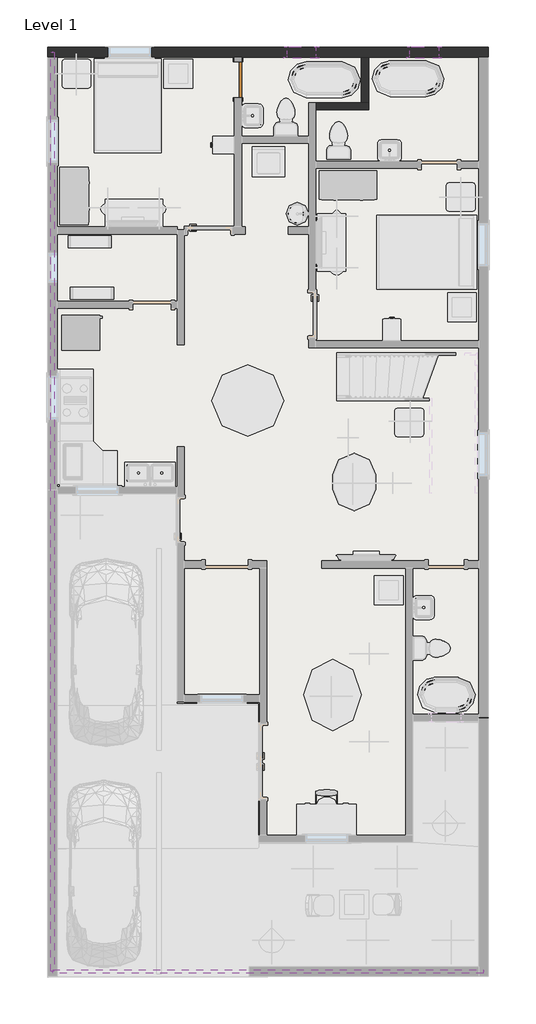
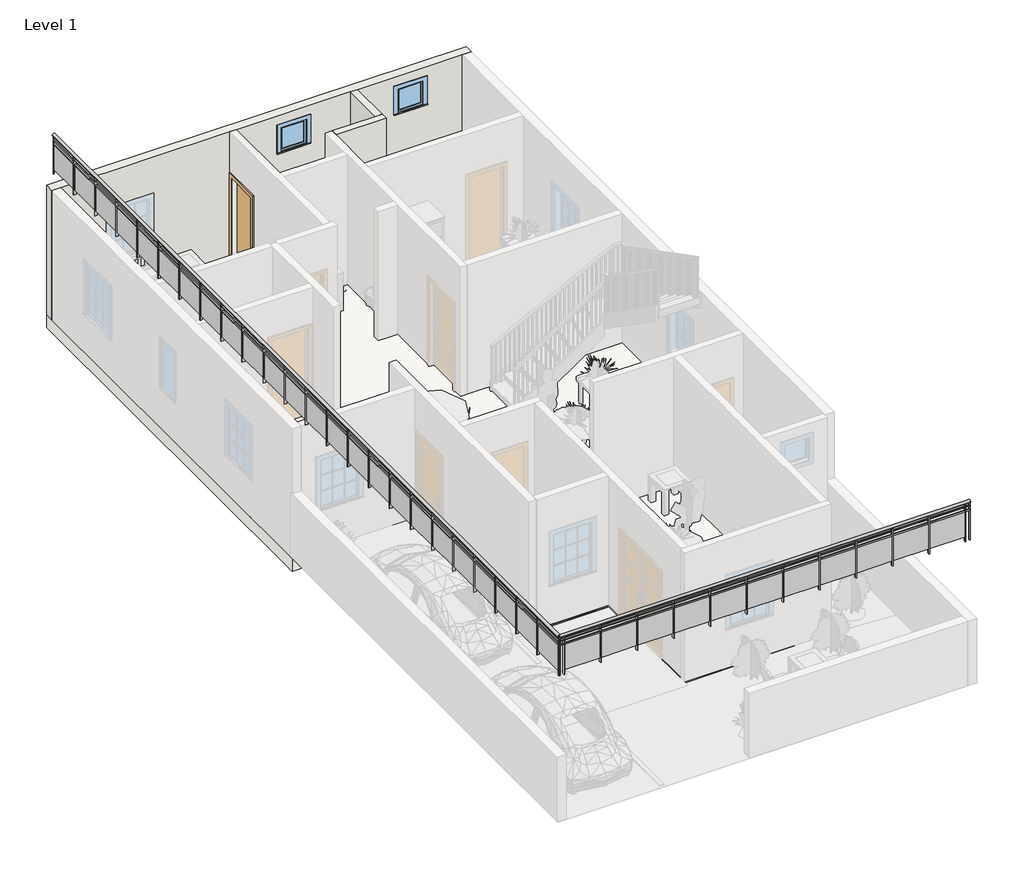
# One storey, part 2 of 4: 3 walls, 2 railings, 2 windows, 1 door, 1 slab.
"""IFC4 building model written with IfcOpenShell, lengths in millimetres."""

from ifc_helpers import new_model, si_unit, point, frame, origin, origin_with_axes, place, context, project, spatial, polyline, ellipse_curve, trimmed, outline, extrude, faceted_brep, transform, mapped, element, save
from ifc_brep_helpers import plane_surface, extruded_surface, advanced_brep
from components import door_255cab33, window_e41d21a6

model = new_model("IFC4")

# Units and contexts
model_context = context("Model", 3, world=origin())
ifc_project = project(units=[si_unit("LENGTHUNIT", "METRE", prefix="MILLI")], contexts=[model_context])

# Site, building, storey
site = spatial("IfcSite", under=ifc_project)
building = spatial("IfcBuilding", under=site)
storey = spatial("IfcBuildingStorey", under=building, Name="Level 1", Elevation=0.0)

# Door
placement = place(None, origin())
door_shape = door_255cab33(model_context)
element("IfcDoor", 1, ObjectType="Single-Flush : 30\" x 80\"", at=placement, inside=storey, context=model_context, shape_type="MappedRepresentation", body=[
    mapped(door_shape, transform((-7763.4976606, 13167.4271763, 0.0), x_axis=(0.0, 1.0, 0.0), y_axis=(-1.0, 0.0, 0.0), z_axis=(0.0, 0.0, 1.0))),
])

# Railings
element("IfcRailing", 2, ObjectType="Glass Panel - Bottom Fill", at=placement, inside=storey, context=model_context, shape_type="SolidModel", body=[
    advanced_brep(
    [(-2556.4976606, -5793.6728237, 4267.2), (-2556.4976606, -5717.4728237, 4267.2), (-11700.4976606, -5793.6728237, 4267.2), (-11700.4976606, -5717.4728237, 4267.2)],
    [
        (0, 1, ellipse_curve(frame((-2556.4976606, -5755.5728237, 4267.2), z_axis=(1.0, 0.0, 0.0), x_axis=(0.0, 1.0, 0.0)), 38.1, 28.575)),
        (1, 0, ellipse_curve(frame((-2556.4976606, -5755.5728237, 4267.2), z_axis=(1.0, 0.0, 0.0), x_axis=(0.0, 1.0, 0.0)), 38.1, 28.575)),
        (2, 3, ellipse_curve(frame((-11700.4976606, -5755.5728237, 4267.2), z_axis=(-1.0, 0.0, 0.0), x_axis=(0.0, 1.0, 0.0)), 38.1, 28.575)),
        (3, 2, ellipse_curve(frame((-11700.4976606, -5755.5728237, 4267.2), z_axis=(-1.0, 0.0, 0.0), x_axis=(0.0, 1.0, 0.0)), 38.1, 28.575)),
        (0, 2),
        (3, 1),
    ],
    [
        plane_surface(frame((-2556.4976606, -5755.5728237, 4267.2), z_axis=(1.0, 0.0, 0.0), x_axis=(0.0, -1.0, 0.0))),
        plane_surface(frame((-11700.4976606, -5755.5728237, 4267.2), z_axis=(-1.0, 0.0, 0.0), x_axis=(0.0, -1.0, 0.0))),
        extruded_surface(trimmed(ellipse_curve(frame((-11700.4976606, -5755.5728237, 4267.2), z_axis=(1.0, 0.0, 0.0), x_axis=(0.0, 1.0, 0.0)), 38.1, 28.575), [point((-11700.4976606, -5793.6728237, 4267.2))], [point((-11700.4976606, -5717.4728237, 4267.2))], True, "CARTESIAN"), (9144.0, 0.0, 0.0), 9144.0),
        extruded_surface(trimmed(ellipse_curve(frame((-11700.4976606, -5755.5728237, 4267.2), z_axis=(1.0, 0.0, 0.0), x_axis=(0.0, 1.0, 0.0)), 38.1, 28.575), [point((-11700.4976606, -5717.4728237, 4267.2))], [point((-11700.4976606, -5793.6728237, 4267.2))], True, "CARTESIAN"), (9144.0, 0.0, 0.0), 9144.0),
    ],
    [
        (0, [[1, 2]]),
        (1, [[3, 4]]),
        (2, [[-1, 5, -4, 6]]),
        (3, [[-2, -6, -3, -5]]),
    ],
),
    extrude(outline(polyline([(-2556.4976606, -5742.8728237), (-2556.4976606, -5768.2728237), (-11700.4976606, -5768.2728237), (-11700.4976606, -5742.8728237), (-2556.4976606, -5742.8728237)])), frame((0.0, 0.0, 4152.9), z_axis=(0.0, 0.0, 1.0), x_axis=(1.0, 0.0, 0.0)), (0.0, 0.0, 1.0), 25.4),
    extrude(outline(polyline([(-2556.4976606, -5742.8728237), (-2556.4976606, -5768.2728237), (-11700.4976606, -5768.2728237), (-11700.4976606, -5742.8728237), (-2556.4976606, -5742.8728237)])), frame((0.0, 0.0, 4051.3), z_axis=(0.0, 0.0, 1.0), x_axis=(1.0, 0.0, 0.0)), (0.0, 0.0, 1.0), 25.4),
    extrude(outline(polyline([(-11592.5476606, -5730.1728237), (-11592.5476606, -5780.9728237), (-11605.2476606, -5780.9728237), (-11605.2476606, -5730.1728237), (-11592.5476606, -5730.1728237)])), frame((0.0, 0.0, 3352.8), z_axis=(0.0, 0.0, 1.0), x_axis=(1.0, 0.0, 0.0)), (0.0, 0.0, 1.0), 885.6788223),
    extrude(outline(polyline([(-10786.0976606, -5762.1079807), (-11598.8976606, -5762.1079807), (-11598.8976606, -5755.7579807), (-10786.0976606, -5755.7579807), (-10786.0976606, -5762.1079807)])), frame((0.0, 0.0, 3454.4), z_axis=(0.0, 0.0, 1.0), x_axis=(1.0, 0.0, 0.0)), (0.0, 0.0, 1.0), 596.9),
    extrude(outline(polyline([(-10779.7476606, -5730.1728237), (-10779.7476606, -5780.9728237), (-10792.4476606, -5780.9728237), (-10792.4476606, -5730.1728237), (-10779.7476606, -5730.1728237)])), frame((0.0, 0.0, 3352.8), z_axis=(0.0, 0.0, 1.0), x_axis=(1.0, 0.0, 0.0)), (0.0, 0.0, 1.0), 885.6788223),
    extrude(outline(polyline([(-9973.2976606, -5762.1079807), (-10786.0976606, -5762.1079807), (-10786.0976606, -5755.7579807), (-9973.2976606, -5755.7579807), (-9973.2976606, -5762.1079807)])), frame((0.0, 0.0, 3454.4), z_axis=(0.0, 0.0, 1.0), x_axis=(1.0, 0.0, 0.0)), (0.0, 0.0, 1.0), 596.9),
    extrude(outline(polyline([(-9966.9476606, -5730.1728237), (-9966.9476606, -5780.9728237), (-9979.6476606, -5780.9728237), (-9979.6476606, -5730.1728237), (-9966.9476606, -5730.1728237)])), frame((0.0, 0.0, 3352.8), z_axis=(0.0, 0.0, 1.0), x_axis=(1.0, 0.0, 0.0)), (0.0, 0.0, 1.0), 885.6788223),
    extrude(outline(polyline([(-9160.4976606, -5762.1079807), (-9973.2976606, -5762.1079807), (-9973.2976606, -5755.7579807), (-9160.4976606, -5755.7579807), (-9160.4976606, -5762.1079807)])), frame((0.0, 0.0, 3454.4), z_axis=(0.0, 0.0, 1.0), x_axis=(1.0, 0.0, 0.0)), (0.0, 0.0, 1.0), 596.9),
    extrude(outline(polyline([(-9154.1476606, -5730.1728237), (-9154.1476606, -5780.9728237), (-9166.8476606, -5780.9728237), (-9166.8476606, -5730.1728237), (-9154.1476606, -5730.1728237)])), frame((0.0, 0.0, 3352.8), z_axis=(0.0, 0.0, 1.0), x_axis=(1.0, 0.0, 0.0)), (0.0, 0.0, 1.0), 885.6788223),
    extrude(outline(polyline([(-8347.6976606, -5762.1079807), (-9160.4976606, -5762.1079807), (-9160.4976606, -5755.7579807), (-8347.6976606, -5755.7579807), (-8347.6976606, -5762.1079807)])), frame((0.0, 0.0, 3454.4), z_axis=(0.0, 0.0, 1.0), x_axis=(1.0, 0.0, 0.0)), (0.0, 0.0, 1.0), 596.9),
    extrude(outline(polyline([(-8341.3476606, -5730.1728237), (-8341.3476606, -5780.9728237), (-8354.0476606, -5780.9728237), (-8354.0476606, -5730.1728237), (-8341.3476606, -5730.1728237)])), frame((0.0, 0.0, 3352.8), z_axis=(0.0, 0.0, 1.0), x_axis=(1.0, 0.0, 0.0)), (0.0, 0.0, 1.0), 885.6788223),
    extrude(outline(polyline([(-7534.8976606, -5762.1079807), (-8347.6976606, -5762.1079807), (-8347.6976606, -5755.7579807), (-7534.8976606, -5755.7579807), (-7534.8976606, -5762.1079807)])), frame((0.0, 0.0, 3454.4), z_axis=(0.0, 0.0, 1.0), x_axis=(1.0, 0.0, 0.0)), (0.0, 0.0, 1.0), 596.9),
    extrude(outline(polyline([(-7528.5476606, -5730.1728237), (-7528.5476606, -5780.9728237), (-7541.2476606, -5780.9728237), (-7541.2476606, -5730.1728237), (-7528.5476606, -5730.1728237)])), frame((0.0, 0.0, 3352.8), z_axis=(0.0, 0.0, 1.0), x_axis=(1.0, 0.0, 0.0)), (0.0, 0.0, 1.0), 885.6788223),
    extrude(outline(polyline([(-6722.0976606, -5762.1079807), (-7534.8976606, -5762.1079807), (-7534.8976606, -5755.7579807), (-6722.0976606, -5755.7579807), (-6722.0976606, -5762.1079807)])), frame((0.0, 0.0, 3454.4), z_axis=(0.0, 0.0, 1.0), x_axis=(1.0, 0.0, 0.0)), (0.0, 0.0, 1.0), 596.9),
    extrude(outline(polyline([(-6715.7476606, -5730.1728237), (-6715.7476606, -5780.9728237), (-6728.4476606, -5780.9728237), (-6728.4476606, -5730.1728237), (-6715.7476606, -5730.1728237)])), frame((0.0, 0.0, 3352.8), z_axis=(0.0, 0.0, 1.0), x_axis=(1.0, 0.0, 0.0)), (0.0, 0.0, 1.0), 885.6788223),
    extrude(outline(polyline([(-5909.2976606, -5762.1079807), (-6722.0976606, -5762.1079807), (-6722.0976606, -5755.7579807), (-5909.2976606, -5755.7579807), (-5909.2976606, -5762.1079807)])), frame((0.0, 0.0, 3454.4), z_axis=(0.0, 0.0, 1.0), x_axis=(1.0, 0.0, 0.0)), (0.0, 0.0, 1.0), 596.9),
    extrude(outline(polyline([(-5902.9476606, -5730.1728237), (-5902.9476606, -5780.9728237), (-5915.6476606, -5780.9728237), (-5915.6476606, -5730.1728237), (-5902.9476606, -5730.1728237)])), frame((0.0, 0.0, 3352.8), z_axis=(0.0, 0.0, 1.0), x_axis=(1.0, 0.0, 0.0)), (0.0, 0.0, 1.0), 885.6788223),
    extrude(outline(polyline([(-5096.4976606, -5762.1079807), (-5909.2976606, -5762.1079807), (-5909.2976606, -5755.7579807), (-5096.4976606, -5755.7579807), (-5096.4976606, -5762.1079807)])), frame((0.0, 0.0, 3454.4), z_axis=(0.0, 0.0, 1.0), x_axis=(1.0, 0.0, 0.0)), (0.0, 0.0, 1.0), 596.9),
    extrude(outline(polyline([(-5090.1476606, -5730.1728237), (-5090.1476606, -5780.9728237), (-5102.8476606, -5780.9728237), (-5102.8476606, -5730.1728237), (-5090.1476606, -5730.1728237)])), frame((0.0, 0.0, 3352.8), z_axis=(0.0, 0.0, 1.0), x_axis=(1.0, 0.0, 0.0)), (0.0, 0.0, 1.0), 885.6788223),
    extrude(outline(polyline([(-4283.6976606, -5762.1079807), (-5096.4976606, -5762.1079807), (-5096.4976606, -5755.7579807), (-4283.6976606, -5755.7579807), (-4283.6976606, -5762.1079807)])), frame((0.0, 0.0, 3454.4), z_axis=(0.0, 0.0, 1.0), x_axis=(1.0, 0.0, 0.0)), (0.0, 0.0, 1.0), 596.9),
    extrude(outline(polyline([(-4277.3476606, -5730.1728237), (-4277.3476606, -5780.9728237), (-4290.0476606, -5780.9728237), (-4290.0476606, -5730.1728237), (-4277.3476606, -5730.1728237)])), frame((0.0, 0.0, 3352.8), z_axis=(0.0, 0.0, 1.0), x_axis=(1.0, 0.0, 0.0)), (0.0, 0.0, 1.0), 885.6788223),
    extrude(outline(polyline([(-3470.8976606, -5762.1079807), (-4283.6976606, -5762.1079807), (-4283.6976606, -5755.7579807), (-3470.8976606, -5755.7579807), (-3470.8976606, -5762.1079807)])), frame((0.0, 0.0, 3454.4), z_axis=(0.0, 0.0, 1.0), x_axis=(1.0, 0.0, 0.0)), (0.0, 0.0, 1.0), 596.9),
    extrude(outline(polyline([(-3464.5476606, -5730.1728237), (-3464.5476606, -5780.9728237), (-3477.2476606, -5780.9728237), (-3477.2476606, -5730.1728237), (-3464.5476606, -5730.1728237)])), frame((0.0, 0.0, 3352.8), z_axis=(0.0, 0.0, 1.0), x_axis=(1.0, 0.0, 0.0)), (0.0, 0.0, 1.0), 885.6788223),
    extrude(outline(polyline([(-2658.0976606, -5762.1079807), (-3470.8976606, -5762.1079807), (-3470.8976606, -5755.7579807), (-2658.0976606, -5755.7579807), (-2658.0976606, -5762.1079807)])), frame((0.0, 0.0, 3454.4), z_axis=(0.0, 0.0, 1.0), x_axis=(1.0, 0.0, 0.0)), (0.0, 0.0, 1.0), 596.9),
    extrude(outline(polyline([(-2651.7476606, -5730.1728237), (-2651.7476606, -5780.9728237), (-2664.4476606, -5780.9728237), (-2664.4476606, -5730.1728237), (-2651.7476606, -5730.1728237)])), frame((0.0, 0.0, 3352.8), z_axis=(0.0, 0.0, 1.0), x_axis=(1.0, 0.0, 0.0)), (0.0, 0.0, 1.0), 885.6788223),
    extrude(outline(polyline([(-11687.7976606, -5746.0478237), (-11687.7976606, -5765.0978237), (-11706.8476606, -5765.0978237), (-11706.8476606, -5746.0478237), (-11687.7976606, -5746.0478237)])), frame((0.0, 0.0, 3352.8), z_axis=(0.0, 0.0, 1.0), x_axis=(1.0, 0.0, 0.0)), (0.0, 0.0, 1.0), 885.6788223),
    extrude(outline(polyline([(-2550.1476606, -5746.0478237), (-2550.1476606, -5765.0978237), (-2569.1976606, -5765.0978237), (-2569.1976606, -5746.0478237), (-2550.1476606, -5746.0478237)])), frame((0.0, 0.0, 3352.8), z_axis=(0.0, 0.0, 1.0), x_axis=(1.0, 0.0, 0.0)), (0.0, 0.0, 1.0), 885.6788223),
])
element("IfcRailing", 3, ObjectType="Glass Panel - Bottom Fill", at=placement, inside=storey, context=model_context, shape_type="SolidModel", body=[
    advanced_brep(
    [(-11738.5976606, -5755.5728237, 4267.2), (-11662.3976606, -5755.5728237, 4267.2), (-11738.5976606, 13751.6271763, 4267.2), (-11662.3976606, 13751.6271763, 4267.2)],
    [
        (0, 1, ellipse_curve(frame((-11700.4976606, -5755.5728237, 4267.2), z_axis=(0.0, -1.0, 0.0), x_axis=(1.0, 0.0, 0.0)), 38.1, 28.575)),
        (1, 0, ellipse_curve(frame((-11700.4976606, -5755.5728237, 4267.2), z_axis=(0.0, -1.0, 0.0), x_axis=(1.0, 0.0, 0.0)), 38.1, 28.575)),
        (2, 3, ellipse_curve(frame((-11700.4976606, 13751.6271763, 4267.2), z_axis=(0.0, 1.0, 0.0), x_axis=(1.0, 0.0, 0.0)), 38.1, 28.575)),
        (3, 2, ellipse_curve(frame((-11700.4976606, 13751.6271763, 4267.2), z_axis=(0.0, 1.0, 0.0), x_axis=(1.0, 0.0, 0.0)), 38.1, 28.575)),
        (0, 2),
        (3, 1),
    ],
    [
        plane_surface(frame((-11700.4976606, -5755.5728237, 4267.2), z_axis=(0.0, -1.0, 0.0), x_axis=(0.0, 0.0, 1.0))),
        plane_surface(frame((-11700.4976606, 13751.6271763, 4267.2), z_axis=(0.0, 1.0, 0.0), x_axis=(0.0, 0.0, 1.0))),
        extruded_surface(trimmed(ellipse_curve(frame((-11700.4976606, 13751.6271763, 4267.2), z_axis=(0.0, -1.0, 0.0), x_axis=(1.0, 0.0, 0.0)), 38.1, 28.575), [point((-11738.5976606, 13751.6271763, 4267.2))], [point((-11662.3976606, 13751.6271763, 4267.2))], True, "CARTESIAN"), (0.0, -19507.2, 0.0), 19507.2),
        extruded_surface(trimmed(ellipse_curve(frame((-11700.4976606, 13751.6271763, 4267.2), z_axis=(0.0, -1.0, 0.0), x_axis=(1.0, 0.0, 0.0)), 38.1, 28.575), [point((-11662.3976606, 13751.6271763, 4267.2))], [point((-11738.5976606, 13751.6271763, 4267.2))], True, "CARTESIAN"), (0.0, -19507.2, 0.0), 19507.2),
    ],
    [
        (0, [[1, 2]]),
        (1, [[3, 4]]),
        (2, [[-1, 5, -4, 6]]),
        (3, [[-2, -6, -3, -5]]),
    ],
),
    extrude(outline(polyline([(-11687.7976606, -5755.5728237), (-11713.1976606, -5755.5728237), (-11713.1976606, 13751.6271763), (-11687.7976606, 13751.6271763), (-11687.7976606, -5755.5728237)])), frame((0.0, 0.0, 4152.9), z_axis=(0.0, 0.0, 1.0), x_axis=(1.0, 0.0, 0.0)), (0.0, 0.0, 1.0), 25.4),
    extrude(outline(polyline([(-11687.7976606, -5755.5728237), (-11713.1976606, -5755.5728237), (-11713.1976606, 13751.6271763), (-11687.7976606, 13751.6271763), (-11687.7976606, -5755.5728237)])), frame((0.0, 0.0, 4051.3), z_axis=(0.0, 0.0, 1.0), x_axis=(1.0, 0.0, 0.0)), (0.0, 0.0, 1.0), 25.4),
    extrude(outline(polyline([(-11707.0328177, 12938.8271763), (-11707.0328177, 13751.6271763), (-11700.6828177, 13751.6271763), (-11700.6828177, 12938.8271763), (-11707.0328177, 12938.8271763)])), frame((0.0, 0.0, 3454.4), z_axis=(0.0, 0.0, 1.0), x_axis=(1.0, 0.0, 0.0)), (0.0, 0.0, 1.0), 596.9),
    extrude(outline(polyline([(-11675.0976606, 12932.4771763), (-11725.8976606, 12932.4771763), (-11725.8976606, 12945.1771763), (-11675.0976606, 12945.1771763), (-11675.0976606, 12932.4771763)])), frame((0.0, 0.0, 3352.8), z_axis=(0.0, 0.0, 1.0), x_axis=(1.0, 0.0, 0.0)), (0.0, 0.0, 1.0), 885.6788223),
    extrude(outline(polyline([(-11707.0328177, 12126.0271763), (-11707.0328177, 12938.8271763), (-11700.6828177, 12938.8271763), (-11700.6828177, 12126.0271763), (-11707.0328177, 12126.0271763)])), frame((0.0, 0.0, 3454.4), z_axis=(0.0, 0.0, 1.0), x_axis=(1.0, 0.0, 0.0)), (0.0, 0.0, 1.0), 596.9),
    extrude(outline(polyline([(-11675.0976606, 12119.6771763), (-11725.8976606, 12119.6771763), (-11725.8976606, 12132.3771763), (-11675.0976606, 12132.3771763), (-11675.0976606, 12119.6771763)])), frame((0.0, 0.0, 3352.8), z_axis=(0.0, 0.0, 1.0), x_axis=(1.0, 0.0, 0.0)), (0.0, 0.0, 1.0), 885.6788223),
    extrude(outline(polyline([(-11707.0328177, 11313.2271763), (-11707.0328177, 12126.0271763), (-11700.6828177, 12126.0271763), (-11700.6828177, 11313.2271763), (-11707.0328177, 11313.2271763)])), frame((0.0, 0.0, 3454.4), z_axis=(0.0, 0.0, 1.0), x_axis=(1.0, 0.0, 0.0)), (0.0, 0.0, 1.0), 596.9),
    extrude(outline(polyline([(-11675.0976606, 11306.8771763), (-11725.8976606, 11306.8771763), (-11725.8976606, 11319.5771763), (-11675.0976606, 11319.5771763), (-11675.0976606, 11306.8771763)])), frame((0.0, 0.0, 3352.8), z_axis=(0.0, 0.0, 1.0), x_axis=(1.0, 0.0, 0.0)), (0.0, 0.0, 1.0), 885.6788223),
    extrude(outline(polyline([(-11707.0328177, 10500.4271763), (-11707.0328177, 11313.2271763), (-11700.6828177, 11313.2271763), (-11700.6828177, 10500.4271763), (-11707.0328177, 10500.4271763)])), frame((0.0, 0.0, 3454.4), z_axis=(0.0, 0.0, 1.0), x_axis=(1.0, 0.0, 0.0)), (0.0, 0.0, 1.0), 596.9),
    extrude(outline(polyline([(-11675.0976606, 10494.0771763), (-11725.8976606, 10494.0771763), (-11725.8976606, 10506.7771763), (-11675.0976606, 10506.7771763), (-11675.0976606, 10494.0771763)])), frame((0.0, 0.0, 3352.8), z_axis=(0.0, 0.0, 1.0), x_axis=(1.0, 0.0, 0.0)), (0.0, 0.0, 1.0), 885.6788223),
    extrude(outline(polyline([(-11707.0328177, 9687.6271763), (-11707.0328177, 10500.4271763), (-11700.6828177, 10500.4271763), (-11700.6828177, 9687.6271763), (-11707.0328177, 9687.6271763)])), frame((0.0, 0.0, 3454.4), z_axis=(0.0, 0.0, 1.0), x_axis=(1.0, 0.0, 0.0)), (0.0, 0.0, 1.0), 596.9),
    extrude(outline(polyline([(-11675.0976606, 9681.2771763), (-11725.8976606, 9681.2771763), (-11725.8976606, 9693.9771763), (-11675.0976606, 9693.9771763), (-11675.0976606, 9681.2771763)])), frame((0.0, 0.0, 3352.8), z_axis=(0.0, 0.0, 1.0), x_axis=(1.0, 0.0, 0.0)), (0.0, 0.0, 1.0), 885.6788223),
    extrude(outline(polyline([(-11707.0328177, 8874.8271763), (-11707.0328177, 9687.6271763), (-11700.6828177, 9687.6271763), (-11700.6828177, 8874.8271763), (-11707.0328177, 8874.8271763)])), frame((0.0, 0.0, 3454.4), z_axis=(0.0, 0.0, 1.0), x_axis=(1.0, 0.0, 0.0)), (0.0, 0.0, 1.0), 596.9),
    extrude(outline(polyline([(-11675.0976606, 8868.4771763), (-11725.8976606, 8868.4771763), (-11725.8976606, 8881.1771763), (-11675.0976606, 8881.1771763), (-11675.0976606, 8868.4771763)])), frame((0.0, 0.0, 3352.8), z_axis=(0.0, 0.0, 1.0), x_axis=(1.0, 0.0, 0.0)), (0.0, 0.0, 1.0), 885.6788223),
    extrude(outline(polyline([(-11707.0328177, 8062.0271763), (-11707.0328177, 8874.8271763), (-11700.6828177, 8874.8271763), (-11700.6828177, 8062.0271763), (-11707.0328177, 8062.0271763)])), frame((0.0, 0.0, 3454.4), z_axis=(0.0, 0.0, 1.0), x_axis=(1.0, 0.0, 0.0)), (0.0, 0.0, 1.0), 596.9),
    extrude(outline(polyline([(-11675.0976606, 8055.6771763), (-11725.8976606, 8055.6771763), (-11725.8976606, 8068.3771763), (-11675.0976606, 8068.3771763), (-11675.0976606, 8055.6771763)])), frame((0.0, 0.0, 3352.8), z_axis=(0.0, 0.0, 1.0), x_axis=(1.0, 0.0, 0.0)), (0.0, 0.0, 1.0), 885.6788223),
    extrude(outline(polyline([(-11707.0328177, 7249.2271763), (-11707.0328177, 8062.0271763), (-11700.6828177, 8062.0271763), (-11700.6828177, 7249.2271763), (-11707.0328177, 7249.2271763)])), frame((0.0, 0.0, 3454.4), z_axis=(0.0, 0.0, 1.0), x_axis=(1.0, 0.0, 0.0)), (0.0, 0.0, 1.0), 596.9),
    extrude(outline(polyline([(-11675.0976606, 7242.8771763), (-11725.8976606, 7242.8771763), (-11725.8976606, 7255.5771763), (-11675.0976606, 7255.5771763), (-11675.0976606, 7242.8771763)])), frame((0.0, 0.0, 3352.8), z_axis=(0.0, 0.0, 1.0), x_axis=(1.0, 0.0, 0.0)), (0.0, 0.0, 1.0), 885.6788223),
    extrude(outline(polyline([(-11707.0328177, 6436.4271763), (-11707.0328177, 7249.2271763), (-11700.6828177, 7249.2271763), (-11700.6828177, 6436.4271763), (-11707.0328177, 6436.4271763)])), frame((0.0, 0.0, 3454.4), z_axis=(0.0, 0.0, 1.0), x_axis=(1.0, 0.0, 0.0)), (0.0, 0.0, 1.0), 596.9),
    extrude(outline(polyline([(-11675.0976606, 6430.0771763), (-11725.8976606, 6430.0771763), (-11725.8976606, 6442.7771763), (-11675.0976606, 6442.7771763), (-11675.0976606, 6430.0771763)])), frame((0.0, 0.0, 3352.8), z_axis=(0.0, 0.0, 1.0), x_axis=(1.0, 0.0, 0.0)), (0.0, 0.0, 1.0), 885.6788223),
    extrude(outline(polyline([(-11707.0328177, 5623.6271763), (-11707.0328177, 6436.4271763), (-11700.6828177, 6436.4271763), (-11700.6828177, 5623.6271763), (-11707.0328177, 5623.6271763)])), frame((0.0, 0.0, 3454.4), z_axis=(0.0, 0.0, 1.0), x_axis=(1.0, 0.0, 0.0)), (0.0, 0.0, 1.0), 596.9),
    extrude(outline(polyline([(-11675.0976606, 5617.2771763), (-11725.8976606, 5617.2771763), (-11725.8976606, 5629.9771763), (-11675.0976606, 5629.9771763), (-11675.0976606, 5617.2771763)])), frame((0.0, 0.0, 3352.8), z_axis=(0.0, 0.0, 1.0), x_axis=(1.0, 0.0, 0.0)), (0.0, 0.0, 1.0), 885.6788223),
    extrude(outline(polyline([(-11707.0328177, 4810.8271763), (-11707.0328177, 5623.6271763), (-11700.6828177, 5623.6271763), (-11700.6828177, 4810.8271763), (-11707.0328177, 4810.8271763)])), frame((0.0, 0.0, 3454.4), z_axis=(0.0, 0.0, 1.0), x_axis=(1.0, 0.0, 0.0)), (0.0, 0.0, 1.0), 596.9),
    extrude(outline(polyline([(-11675.0976606, 4804.4771763), (-11725.8976606, 4804.4771763), (-11725.8976606, 4817.1771763), (-11675.0976606, 4817.1771763), (-11675.0976606, 4804.4771763)])), frame((0.0, 0.0, 3352.8), z_axis=(0.0, 0.0, 1.0), x_axis=(1.0, 0.0, 0.0)), (0.0, 0.0, 1.0), 885.6788223),
    extrude(outline(polyline([(-11707.0328177, 3998.0271763), (-11707.0328177, 4810.8271763), (-11700.6828177, 4810.8271763), (-11700.6828177, 3998.0271763), (-11707.0328177, 3998.0271763)])), frame((0.0, 0.0, 3454.4), z_axis=(0.0, 0.0, 1.0), x_axis=(1.0, 0.0, 0.0)), (0.0, 0.0, 1.0), 596.9),
    extrude(outline(polyline([(-11675.0976606, 3991.6771763), (-11725.8976606, 3991.6771763), (-11725.8976606, 4004.3771763), (-11675.0976606, 4004.3771763), (-11675.0976606, 3991.6771763)])), frame((0.0, 0.0, 3352.8), z_axis=(0.0, 0.0, 1.0), x_axis=(1.0, 0.0, 0.0)), (0.0, 0.0, 1.0), 885.6788223),
    extrude(outline(polyline([(-11707.0328177, 3185.2271763), (-11707.0328177, 3998.0271763), (-11700.6828177, 3998.0271763), (-11700.6828177, 3185.2271763), (-11707.0328177, 3185.2271763)])), frame((0.0, 0.0, 3454.4), z_axis=(0.0, 0.0, 1.0), x_axis=(1.0, 0.0, 0.0)), (0.0, 0.0, 1.0), 596.9),
    extrude(outline(polyline([(-11675.0976606, 3178.8771763), (-11725.8976606, 3178.8771763), (-11725.8976606, 3191.5771763), (-11675.0976606, 3191.5771763), (-11675.0976606, 3178.8771763)])), frame((0.0, 0.0, 3352.8), z_axis=(0.0, 0.0, 1.0), x_axis=(1.0, 0.0, 0.0)), (0.0, 0.0, 1.0), 885.6788223),
    extrude(outline(polyline([(-11707.0328177, 2372.4271763), (-11707.0328177, 3185.2271763), (-11700.6828177, 3185.2271763), (-11700.6828177, 2372.4271763), (-11707.0328177, 2372.4271763)])), frame((0.0, 0.0, 3454.4), z_axis=(0.0, 0.0, 1.0), x_axis=(1.0, 0.0, 0.0)), (0.0, 0.0, 1.0), 596.9),
    extrude(outline(polyline([(-11675.0976606, 2366.0771763), (-11725.8976606, 2366.0771763), (-11725.8976606, 2378.7771763), (-11675.0976606, 2378.7771763), (-11675.0976606, 2366.0771763)])), frame((0.0, 0.0, 3352.8), z_axis=(0.0, 0.0, 1.0), x_axis=(1.0, 0.0, 0.0)), (0.0, 0.0, 1.0), 885.6788223),
    extrude(outline(polyline([(-11707.0328177, 1559.6271763), (-11707.0328177, 2372.4271763), (-11700.6828177, 2372.4271763), (-11700.6828177, 1559.6271763), (-11707.0328177, 1559.6271763)])), frame((0.0, 0.0, 3454.4), z_axis=(0.0, 0.0, 1.0), x_axis=(1.0, 0.0, 0.0)), (0.0, 0.0, 1.0), 596.9),
    extrude(outline(polyline([(-11675.0976606, 1553.2771763), (-11725.8976606, 1553.2771763), (-11725.8976606, 1565.9771763), (-11675.0976606, 1565.9771763), (-11675.0976606, 1553.2771763)])), frame((0.0, 0.0, 3352.8), z_axis=(0.0, 0.0, 1.0), x_axis=(1.0, 0.0, 0.0)), (0.0, 0.0, 1.0), 885.6788223),
    extrude(outline(polyline([(-11707.0328177, 746.8271763), (-11707.0328177, 1559.6271763), (-11700.6828177, 1559.6271763), (-11700.6828177, 746.8271763), (-11707.0328177, 746.8271763)])), frame((0.0, 0.0, 3454.4), z_axis=(0.0, 0.0, 1.0), x_axis=(1.0, 0.0, 0.0)), (0.0, 0.0, 1.0), 596.9),
    extrude(outline(polyline([(-11675.0976606, 740.4771763), (-11725.8976606, 740.4771763), (-11725.8976606, 753.1771763), (-11675.0976606, 753.1771763), (-11675.0976606, 740.4771763)])), frame((0.0, 0.0, 3352.8), z_axis=(0.0, 0.0, 1.0), x_axis=(1.0, 0.0, 0.0)), (0.0, 0.0, 1.0), 885.6788223),
    extrude(outline(polyline([(-11707.0328177, -65.9728237), (-11707.0328177, 746.8271763), (-11700.6828177, 746.8271763), (-11700.6828177, -65.9728237), (-11707.0328177, -65.9728237)])), frame((0.0, 0.0, 3454.4), z_axis=(0.0, 0.0, 1.0), x_axis=(1.0, 0.0, 0.0)), (0.0, 0.0, 1.0), 596.9),
    extrude(outline(polyline([(-11675.0976606, -72.3228237), (-11725.8976606, -72.3228237), (-11725.8976606, -59.6228237), (-11675.0976606, -59.6228237), (-11675.0976606, -72.3228237)])), frame((0.0, 0.0, 3352.8), z_axis=(0.0, 0.0, 1.0), x_axis=(1.0, 0.0, 0.0)), (0.0, 0.0, 1.0), 885.6788223),
    extrude(outline(polyline([(-11707.0328177, -878.7728237), (-11707.0328177, -65.9728237), (-11700.6828177, -65.9728237), (-11700.6828177, -878.7728237), (-11707.0328177, -878.7728237)])), frame((0.0, 0.0, 3454.4), z_axis=(0.0, 0.0, 1.0), x_axis=(1.0, 0.0, 0.0)), (0.0, 0.0, 1.0), 596.9),
    extrude(outline(polyline([(-11675.0976606, -885.1228237), (-11725.8976606, -885.1228237), (-11725.8976606, -872.4228237), (-11675.0976606, -872.4228237), (-11675.0976606, -885.1228237)])), frame((0.0, 0.0, 3352.8), z_axis=(0.0, 0.0, 1.0), x_axis=(1.0, 0.0, 0.0)), (0.0, 0.0, 1.0), 885.6788223),
    extrude(outline(polyline([(-11707.0328177, -1691.5728237), (-11707.0328177, -878.7728237), (-11700.6828177, -878.7728237), (-11700.6828177, -1691.5728237), (-11707.0328177, -1691.5728237)])), frame((0.0, 0.0, 3454.4), z_axis=(0.0, 0.0, 1.0), x_axis=(1.0, 0.0, 0.0)), (0.0, 0.0, 1.0), 596.9),
    extrude(outline(polyline([(-11675.0976606, -1697.9228237), (-11725.8976606, -1697.9228237), (-11725.8976606, -1685.2228237), (-11675.0976606, -1685.2228237), (-11675.0976606, -1697.9228237)])), frame((0.0, 0.0, 3352.8), z_axis=(0.0, 0.0, 1.0), x_axis=(1.0, 0.0, 0.0)), (0.0, 0.0, 1.0), 885.6788223),
    extrude(outline(polyline([(-11707.0328177, -2504.3728237), (-11707.0328177, -1691.5728237), (-11700.6828177, -1691.5728237), (-11700.6828177, -2504.3728237), (-11707.0328177, -2504.3728237)])), frame((0.0, 0.0, 3454.4), z_axis=(0.0, 0.0, 1.0), x_axis=(1.0, 0.0, 0.0)), (0.0, 0.0, 1.0), 596.9),
    extrude(outline(polyline([(-11675.0976606, -2510.7228237), (-11725.8976606, -2510.7228237), (-11725.8976606, -2498.0228237), (-11675.0976606, -2498.0228237), (-11675.0976606, -2510.7228237)])), frame((0.0, 0.0, 3352.8), z_axis=(0.0, 0.0, 1.0), x_axis=(1.0, 0.0, 0.0)), (0.0, 0.0, 1.0), 885.6788223),
    extrude(outline(polyline([(-11707.0328177, -3317.1728237), (-11707.0328177, -2504.3728237), (-11700.6828177, -2504.3728237), (-11700.6828177, -3317.1728237), (-11707.0328177, -3317.1728237)])), frame((0.0, 0.0, 3454.4), z_axis=(0.0, 0.0, 1.0), x_axis=(1.0, 0.0, 0.0)), (0.0, 0.0, 1.0), 596.9),
    extrude(outline(polyline([(-11675.0976606, -3323.5228237), (-11725.8976606, -3323.5228237), (-11725.8976606, -3310.8228237), (-11675.0976606, -3310.8228237), (-11675.0976606, -3323.5228237)])), frame((0.0, 0.0, 3352.8), z_axis=(0.0, 0.0, 1.0), x_axis=(1.0, 0.0, 0.0)), (0.0, 0.0, 1.0), 885.6788223),
    extrude(outline(polyline([(-11707.0328177, -4129.9728237), (-11707.0328177, -3317.1728237), (-11700.6828177, -3317.1728237), (-11700.6828177, -4129.9728237), (-11707.0328177, -4129.9728237)])), frame((0.0, 0.0, 3454.4), z_axis=(0.0, 0.0, 1.0), x_axis=(1.0, 0.0, 0.0)), (0.0, 0.0, 1.0), 596.9),
    extrude(outline(polyline([(-11675.0976606, -4136.3228237), (-11725.8976606, -4136.3228237), (-11725.8976606, -4123.6228237), (-11675.0976606, -4123.6228237), (-11675.0976606, -4136.3228237)])), frame((0.0, 0.0, 3352.8), z_axis=(0.0, 0.0, 1.0), x_axis=(1.0, 0.0, 0.0)), (0.0, 0.0, 1.0), 885.6788223),
    extrude(outline(polyline([(-11707.0328177, -4942.7728237), (-11707.0328177, -4129.9728237), (-11700.6828177, -4129.9728237), (-11700.6828177, -4942.7728237), (-11707.0328177, -4942.7728237)])), frame((0.0, 0.0, 3454.4), z_axis=(0.0, 0.0, 1.0), x_axis=(1.0, 0.0, 0.0)), (0.0, 0.0, 1.0), 596.9),
    extrude(outline(polyline([(-11675.0976606, -4949.1228237), (-11725.8976606, -4949.1228237), (-11725.8976606, -4936.4228237), (-11675.0976606, -4936.4228237), (-11675.0976606, -4949.1228237)])), frame((0.0, 0.0, 3352.8), z_axis=(0.0, 0.0, 1.0), x_axis=(1.0, 0.0, 0.0)), (0.0, 0.0, 1.0), 885.6788223),
    extrude(outline(polyline([(-11707.0328177, -5755.5728237), (-11707.0328177, -4942.7728237), (-11700.6828177, -4942.7728237), (-11700.6828177, -5755.5728237), (-11707.0328177, -5755.5728237)])), frame((0.0, 0.0, 3454.4), z_axis=(0.0, 0.0, 1.0), x_axis=(1.0, 0.0, 0.0)), (0.0, 0.0, 1.0), 596.9),
    extrude(outline(polyline([(-11690.9726606, 13738.9271763), (-11710.0226606, 13738.9271763), (-11710.0226606, 13757.9771763), (-11690.9726606, 13757.9771763), (-11690.9726606, 13738.9271763)])), frame((0.0, 0.0, 3352.8), z_axis=(0.0, 0.0, 1.0), x_axis=(1.0, 0.0, 0.0)), (0.0, 0.0, 1.0), 885.6788223),
    extrude(outline(polyline([(-11690.9726606, -5761.9228237), (-11710.0226606, -5761.9228237), (-11710.0226606, -5742.8728237), (-11690.9726606, -5742.8728237), (-11690.9726606, -5761.9228237)])), frame((0.0, 0.0, 3352.8), z_axis=(0.0, 0.0, 1.0), x_axis=(1.0, 0.0, 0.0)), (0.0, 0.0, 1.0), 885.6788223),
])

# Slab
element("IfcSlab", 4, ObjectType="Generic - 12\"", at=placement, inside=storey, context=model_context, shape_type="SweptSolid", body=[
    extrude(outline(polyline([(-2454.8976606, 13853.2271763), (-2454.8976606, -446.9728237), (-4055.0976606, -446.9728237), (-4055.0976606, -3012.3728237), (-7318.9976606, -3012.3728237), (-7318.9976606, -65.9728237), (-9058.8976606, -65.9728237), (-9058.8976606, 4379.0271763), (-11802.0976606, 4379.0271763), (-11802.0976606, 13853.2271763), (-2454.8976606, 13853.2271763)])), frame((0.0, 0.0, -304.8), z_axis=(0.0, 0.0, 1.0), x_axis=(1.0, 0.0, 0.0)), (0.0, 0.0, 1.0), 304.8),
])

# Walls
element("IfcWall", 5, ObjectType="Generic - 8\"", at=placement, inside=storey, context=model_context, shape_type="Brep", body=[
    faceted_brep([(-11802.0976606, 13650.0271763, 0.0), (-11598.8976606, 13650.0271763, 0.0), (-7839.6976606, 13650.0271763, 0.0), (-7687.2976606, 13650.0271763, 0.0), (-5147.2976606, 13650.0271763, 0.0), (-4994.8976606, 13650.0271763, 0.0), (-2658.0976606, 13650.0271763, 0.0), (-2454.8976606, 13650.0271763, 0.0), (-2454.8976606, 13650.0271763, 3048.0), (-2658.0976606, 13650.0271763, 3048.0), (-4994.8976606, 13650.0271763, 3048.0), (-5147.2976606, 13650.0271763, 3048.0), (-7687.2976606, 13650.0271763, 3048.0), (-7839.6976606, 13650.0271763, 3048.0), (-11598.8976606, 13650.0271763, 3048.0), (-11802.0976606, 13650.0271763, 3048.0), (-9604.9976606, 13650.0271763, 2133.6), (-9604.9976606, 13650.0271763, 914.4), (-10519.3976606, 13650.0271763, 914.4), (-10519.3976606, 13650.0271763, 2133.6), (-6722.0976606, 13650.0271763, 2768.6), (-6112.4976606, 13650.0271763, 2768.6), (-6112.4976606, 13650.0271763, 2159.0), (-6722.0976606, 13650.0271763, 2159.0), (-4118.5976606, 13650.0271763, 2768.6), (-3508.9976606, 13650.0271763, 2768.6), (-3508.9976606, 13650.0271763, 2159.0), (-4118.5976606, 13650.0271763, 2159.0), (-11802.0976606, 13853.2271763, 0.0), (-11802.0976606, 13853.2271763, 3048.0), (-2454.8976606, 13853.2271763, 3048.0), (-2454.8976606, 13853.2271763, 0.0), (-9604.9976606, 13853.2271763, 2133.6), (-10519.3976606, 13853.2271763, 2133.6), (-10519.3976606, 13853.2271763, 914.4), (-9604.9976606, 13853.2271763, 914.4), (-6722.0976606, 13853.2271763, 2768.6), (-6722.0976606, 13853.2271763, 2159.0), (-6112.4976606, 13853.2271763, 2159.0), (-6112.4976606, 13853.2271763, 2768.6), (-4118.5976606, 13853.2271763, 2768.6), (-4118.5976606, 13853.2271763, 2159.0), (-3508.9976606, 13853.2271763, 2159.0), (-3508.9976606, 13853.2271763, 2768.6)], [[[0, 1, 2, 3, 4, 5, 6, 7, 8, 9, 10, 11, 12, 13, 14, 15], [16, 17, 18, 19], [20, 21, 22, 23], [24, 25, 26, 27]], [[28, 29, 30, 31], [32, 33, 34, 35], [36, 37, 38, 39], [40, 41, 42, 43]], [[7, 6, 5, 4, 3, 2, 1, 0, 28, 31]], [[8, 7, 31, 30]], [[0, 15, 29, 28]], [[17, 16, 32, 35]], [[18, 17, 35, 34]], [[19, 18, 34, 33]], [[16, 19, 33, 32]], [[37, 36, 20, 23]], [[38, 37, 23, 22]], [[39, 38, 22, 21]], [[36, 39, 21, 20]], [[41, 40, 24, 27]], [[42, 41, 27, 26]], [[43, 42, 26, 25]], [[40, 43, 25, 24]], [[15, 14, 13, 12, 11, 10, 9, 8, 30, 29]]]),
])
element("IfcWall", 6, ObjectType="inner 6\"", at=placement, inside=storey, context=model_context, shape_type="Brep", body=[
    faceted_brep([(-6112.4976606, 12532.4271763, 0.0), (-4994.8976606, 12532.4271763, 0.0), (-4994.8976606, 12532.4271763, 3048.0), (-6112.4976606, 12532.4271763, 3048.0), (-6112.4976606, 12684.8271763, 0.0), (-6112.4976606, 12684.8271763, 3048.0), (-5147.2976606, 12684.8271763, 3048.0), (-4994.8976606, 12684.8271763, 3048.0), (-4994.8976606, 12684.8271763, 0.0), (-5147.2976606, 12684.8271763, 0.0)], [[[0, 1, 2, 3]], [[4, 5, 6, 7, 8, 9]], [[1, 0, 4, 9, 8]], [[0, 3, 5, 4]], [[2, 1, 8, 7]], [[3, 2, 7, 6, 5]]]),
])
element("IfcWall", 7, ObjectType="inner 6\"", at=placement, inside=storey, context=model_context, shape_type="SweptSolid", body=[
    extrude(outline(polyline([(-4994.8976606, 13650.0271763), (-4994.8976606, 12684.8271763), (-5147.2976606, 12684.8271763), (-5147.2976606, 13650.0271763), (-4994.8976606, 13650.0271763)])), origin_with_axes(), (0.0, 0.0, 1.0), 3048.0),
])

# Windows
window_shape = window_e41d21a6(model_context)
element("IfcWindow", 8, ObjectType="Transom with Trim : 24\" x 24\"", at=placement, inside=storey, context=model_context, shape_type="MappedRepresentation", body=[
    mapped(window_shape, transform((-6455.3976606, 13751.6271763, 0.0), x_axis=(-1.0, 0.0, 0.0), y_axis=(0.0, -1.0, 0.0), z_axis=(0.0, 0.0, 1.0))),
])
element("IfcWindow", 9, ObjectType="Transom with Trim : 24\" x 24\"", at=placement, inside=storey, context=model_context, shape_type="MappedRepresentation", body=[
    mapped(window_shape, transform((-3851.8976606, 13751.6271763, 0.0), x_axis=(-1.0, 0.0, 0.0), y_axis=(0.0, -1.0, 0.0), z_axis=(0.0, 0.0, 1.0))),
])

save(model, "model.ifc")

# Revit data of these elements
# Type "Single-Flush : 30\" x 80\""
#   Type Mark = "5"
#   Construction Type Id = "MDOOR"
#   Assembly Code = "C1020"
#   Analytic Construction = "Metal"
#   Thickness = 0' - 2"
#   Heat Transfer Coefficient (U) = 0.651978 BTU/(h·ft²·°F)
#   Height = 6' - 8"
#   Trim Projection Ext = 0' - 1"
#   Trim Projection Int = 0' - 1"
#   Trim Width = 0' - 3"
#   Width = 2' - 6"
#   Define Thermal Properties by = 1
#   Door Material = Door - Panel
#   Frame Material = Door - Frame
#   Visual Light Transmittance = 0
#   Solar Heat Gain Coefficient = 0
#   Function = (empty or 0)
#   Wall Closure = (empty or 0)
# Type "Glass Panel - Bottom Fill"
#   Assembly Code = "C2010400"
#   built-in parameter 1008612 = 0.0416667 (stored number, unit not read)
#   built-in parameter 1008611 = 0.0416667 (stored number, unit not read)
#   built-in parameter 1008609 = 0.333333 (stored number, unit not read)
#   built-in parameter 1008604 = 0.166667 (stored number, unit not read)
#   built-in parameter 1008603 = 0.166667 (stored number, unit not read)
#   Railing Height = 3' - 0"
#   built-in parameter 1008630 = 2
#   built-in parameter 1008610 = 2
#   built-in parameter 1008618 = Baluster - Square : 3/4"
# Type "Generic - 12\""
#   Assembly Code = "B1010"
#   Function = 0
#   Layers, outside or top first: 1' - 0" no material (function 1)
# Type "Generic - 8\""
#   Assembly Code = "B2010"
#   Layers, outside or top first: 0' - 8" "Brick, Common" (function 1)
# Type "inner 6\""
#   Assembly Code = "B2010"
#   Layers, outside or top first: 0' - 6" "Brick, Common" (function 1)
# Type "Transom with Trim : 24\" x 24\""
#   Type Mark = "13"
#   Construction Type Id = "GSP4R"
#   Assembly Code = "B2020100"
#   Analytic Construction = "1/8 in Pilkington single glazing"
#   Visual Light Transmittance = 0.9
#   Solar Heat Gain Coefficient = 0.78
#   Heat Transfer Coefficient (U) = 0.6496 BTU/(h·ft²·°F)
#   Height = 2' - 0"
#   Default Sill Height = 7' - 1"
#   Trim Projection - Ext. = 0' - 0 1/2"
#   Trim Projection - Int. = 0' - 0 3/4"
#   Trim Width - Exterior = 0' - 3 1/2"
#   Trim Width - Interior = 0' - 3 1/2"
#   Width = 2' - 0"
#   Window Inset = 0' - 0 3/4"
#   Define Thermal Properties by = 1
#   Glass Pane Material = Glass
#   Sash Material = Sash
#   Trim Exterior Material = Trim
#   Trim Interior Material = Trim
#   Wall Closure = (empty or 0)
# Element 1 (IfcDoor, "Single-Flush : 30\" x 80\"")
#   Phase Created = New Construction
#   Materials on its faces: "Door - Frame", "Door - Panel"
# Elements 2, 3 (IfcRailing, "Glass Panel - Bottom Fill")
#   built-in parameter 1008621 = 11 (stored number, unit not read)
#   Phase Created = New Construction
#   Materials on its faces: "Glass"
# Element 4 (IfcSlab, "Generic - 12\"")
#   Height Offset From Level = 0' - 0"
#   Phase Created = New Construction
#   Materials on its faces: "Default Floor"
# Element 5 (IfcWall, "Generic - 8\"")
#   Top Offset = 0' - 0"
#   Base Offset = 0' - 0"
#   Unconnected Height = 10' - 0"
#   wall height = 10' - 0"
#   Phase Created = New Construction
#   Base Constraint = Level 1
#   Materials on its faces: "Brick, Common"
# Elements 6, 7 (IfcWall, "inner 6\"")
#   Top Offset = 0' - 0"
#   Base Offset = 0' - 0"
#   Unconnected Height = 10' - 0"
#   wall height = 10' - 0"
#   Phase Created = New Construction
#   Base Constraint = Level 1
#   Materials on its faces: "Brick, Common"
# Element 8 (IfcWindow, "Transom with Trim : 24\" x 24\"")
#   Mark = "10"
#   Phase Created = New Construction
#   Materials on its faces: "Sash", "Trim", "Glass"
# Element 9 (IfcWindow, "Transom with Trim : 24\" x 24\"")
#   Mark = "11"
#   Phase Created = New Construction
#   Materials on its faces: "Sash", "Trim", "Glass"
# Materials
#   "Door - Panel": class "Wood", colour RGB 210 159 95, transparency 0
#   "Door - Frame": colour RGB 118 70 51, transparency 0
#   "Brick, Common": class "Masonry", colour RGB 170 98 104, transparency 0, Description = "Common brick", Cost = 0
#   "Glass": class "Glass", colour RGB 0 128 192, transparency 0.75, Description = "Soda Lime Glass", Cost = 0
#   "Sash": class "Wood", colour RGB 224 178 126, transparency 0
#   "Trim": class "Wood", colour RGB 224 178 126, transparency 0
#   "Default Floor": colour RGB 128 128 128, transparency 0
